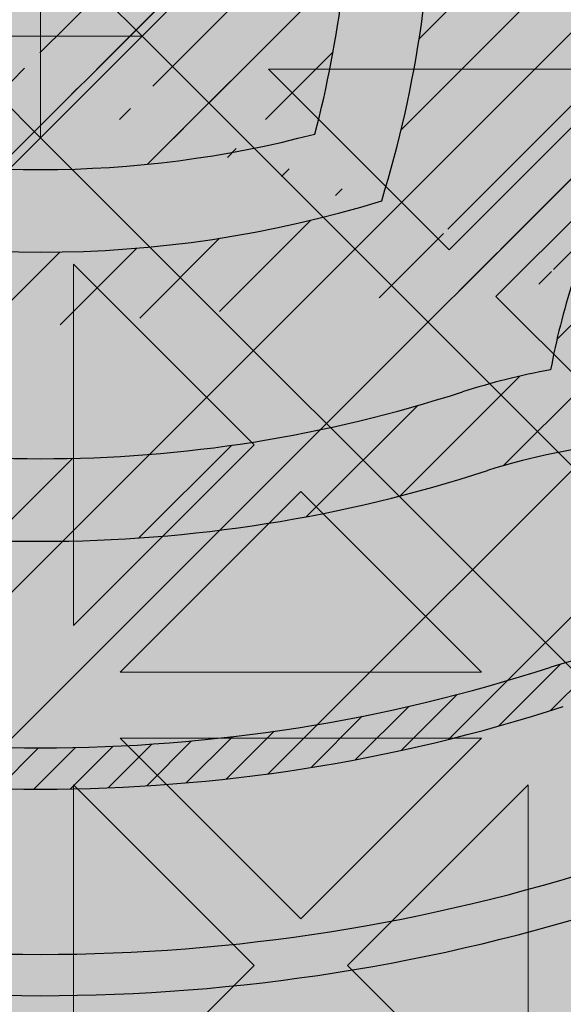
# Model space of a CAD drawing. Units: inches. Extents: x 844 to 2234, y 346 to 1084.
# Tile 54 of 93: x 1869.26 to 1871.357, y 692.527 to 696.327. Entities that reach past the tile are written whole.
import ezdxf

# ---------------------------------------------------------------- set-up
doc = ezdxf.new("R2010")
doc.units = ezdxf.units.IN
doc.header["$MEASUREMENT"] = 0
doc.layers.add('furniture', color=8, linetype='Continuous', lineweight=18)
doc.layers.add('RA-AP-01$0$INT', color=35, linetype='Continuous', lineweight=5)
doc.layers.add('RA-AP-01$0$FURN', color=3, linetype='Continuous')
doc.layers.add('RA-AP-01$0$WOOD', color=64, linetype='Continuous')

# ---------------------------------------------------------------- blocks, each defined once
blk = doc.blocks.new('A$C18D01794')
at = {"layer": 'RA-AP-01$0$INT'}
h = blk.add_hatch(color=256, dxfattribs=at)
h.paths.add_polyline_path([(4.585917135068449, -6.356712009588271), (4.555206456959269, -6.35671200958746), (4.555206456959137, -6.387422687716308), (4.874495778835233, -6.706712009592356), (4.90520645695423, -6.676001331474049)])
h.paths.add_polyline_path([(5.255206456948813, -6.387422687716306), (5.255206456948682, -6.356712009605972), (5.224495778822613, -6.356712009605161), (4.905206456953498, -6.676001331474273), (4.935917135072151, -6.706712009592924)])
h.paths.add_polyline_path([(4.935917135072559, -6.706712009592068), (4.905206456953564, -6.737422687710376), (5.255206456951813, -7.087422687708613), (5.255206456951549, -7.026001331471008)])
h.paths.add_polyline_path([(4.555206456956399, -7.026001331471013), (4.555206456956134, -7.087422687708616), (4.905206456953821, -6.737422687710943), (4.874495778835166, -6.70671200959229)])
h = blk.add_hatch(color=256, dxfattribs=at)
h.paths.add_polyline_path([(4.585917135068448, -6.356712009588273), (4.614201406330596, -6.356712009589021), (4.668846067270487, -6.411356670531338), (4.723490728212344, -6.356712009591912), (4.771774999457151, -6.35671200959319), (4.826419660396886, -6.411356670535356), (4.862780050090322, -6.374996280843536), (4.844495778842715, -6.356712009595112), (4.862780050090411, -6.356712009595595), (4.905206456960182, -6.399138416468211), (4.947632863832445, -6.356712009597838), (4.965917135079675, -6.356712009598322), (4.947632863831759, -6.374996280845421), (4.983993253523576, -6.411356670538857), (5.038637914464627, -6.356712009600247), (5.08692218571208, -6.356712009601523), (5.141566846649976, -6.411356670541852), (5.196211507589851, -6.356712009604411), (5.224495778822615, -6.356712009605161), (4.905206456953975, -6.676001331473793)])
h.paths.add_polyline_path([(4.895206456956031, -6.637717060225675), (4.895206456958921, -6.528427738347902), (4.840561796018589, -6.583072399285802)], flags=16)
h.paths.add_polyline_path([(4.915206456955638, -6.637717060226121), (4.969851117895509, -6.583072399288678), (4.915206456957609, -6.528427738348344)], flags=16)
h.paths.add_polyline_path([(4.826419660395175, -6.568930263661755), (4.881064321335613, -6.514285602723745), (4.771774999456703, -6.514285602720857)], flags=16)
h.paths.add_polyline_path([(4.983993253519558, -6.568930263665262), (5.038637914460456, -6.514285602726792), (4.929348592581548, -6.514285602724816)], flags=16)
h.paths.add_polyline_path([(4.881064321336025, -6.494285602723742), (4.826419660397532, -6.439640941782821), (4.771774999457062, -6.494285602720859)], flags=16)
h.paths.add_polyline_path([(4.929348592582019, -6.494285602724817), (5.038637914460982, -6.494285602726792), (4.983993253522945, -6.439640941786327)], flags=16)
h.paths.add_polyline_path([(4.895206456960191, -6.480143467100443), (4.895206456962115, -6.407422687715913), (4.876922185715016, -6.389138416467584), (4.840561796021581, -6.425498806159401)], flags=16)
h.paths.add_polyline_path([(4.915206456958487, -6.480143467100889), (4.969851117899527, -6.425498806162279), (4.933490728206909, -6.389138416468043), (4.9152064569598, -6.40742268771434)], flags=16)
h.paths.add_polyline_path([(4.757632863832376, -6.480143467096812), (4.812277524772842, -6.425498806158772), (4.757632863834348, -6.370854145217844)], flags=16)
h.paths.add_polyline_path([(4.737632863832376, -6.480143467096286), (4.737632863834348, -6.370854145217375), (4.682988202893906, -6.425498806155385)], flags=16)
h.paths.add_polyline_path([(5.05278005008503, -6.480143467103376), (5.052780050087917, -6.370854145224413), (4.998135389146995, -6.425498806162908)], flags=16)
h.paths.add_polyline_path([(5.072780050085024, -6.480143467103744), (5.127424711025931, -6.42549880616527), (5.072780050087916, -6.370854145224832)], flags=16)
h.paths.add_polyline_path([(4.935917135072783, -6.706712009592292), (5.255206456948811, -6.387422687716309), (5.255206456948932, -6.415706958964177), (5.200561796010279, -6.470351619902839), (5.255206456949403, -6.524996280841948), (5.25520645694961, -6.5732805520894), (5.200561796009787, -6.627925213029239), (5.236922185702417, -6.664285602721864), (5.255206456949919, -6.646001331474357), (5.255206456949998, -6.664285602721898), (5.212780050078687, -6.706712009592262), (5.25520645695036, -6.749138416463932), (5.255206456950438, -6.767422687711313), (5.236922185702424, -6.749138416463297), (5.200561796009796, -6.785498806155928), (5.255206456950753, -6.840143467096874), (5.25520645695096, -6.888427738341682), (5.200561796010322, -6.943072399282328), (5.255206456951428, -6.997717060223427), (5.255206456951547, -7.026001331471006)])
h.paths.add_polyline_path([(5.042988202883395, -6.785498806155427), (5.097632863823085, -6.840143467095101), (5.097632863822622, -6.730854145216193)], flags=16)
h.paths.add_polyline_path([(5.028846067259663, -6.771356670531693), (5.083490728198774, -6.716712009592573), (4.974201406321001, -6.716712009593042)], flags=16)
h.paths.add_polyline_path([(5.117632863823087, -6.840143467095186), (5.172277524762331, -6.785498806155926), (5.11763286382262, -6.730854145216225)], flags=16)
h.paths.add_polyline_path([(5.08349072819877, -6.696712009593886), (5.028846067259652, -6.642067348654775), (4.974201406320998, -6.696712009593438)], flags=16)
h.paths.add_polyline_path([(5.131774999446817, -6.854285602718917), (5.186419660386065, -6.799640941779662), (5.241064321325782, -6.854285602719365)], flags=17)
h.paths.add_polyline_path([(5.131774999446228, -6.716712009592374), (5.186419660386065, -6.771356670532194), (5.222780050079488, -6.734996280838764), (5.204495778832781, -6.716712009592063)], flags=16)
h.paths.add_polyline_path([(5.097632863822613, -6.682569873970264), (5.097632863823061, -6.573280552091354), (5.042988202883383, -6.627925213031044)], flags=16)
h.paths.add_polyline_path([(5.131774999446899, -6.874285602718915), (5.241064321325809, -6.874285602719364), (5.186419660386591, -6.928930263658598)], flags=17)
h.paths.add_polyline_path([(5.131774999446226, -6.696712009594078), (5.204495778830767, -6.696712009594374), (5.22278005007868, -6.67842773834687), (5.186419660386049, -6.642067348654249)], flags=16)
h.paths.add_polyline_path([(5.11763286382262, -6.682569873970225), (5.17227752476232, -6.627925213030515), (5.117632863823064, -6.573280552091267)], flags=16)
h.paths.add_polyline_path([(5.186419660386069, -6.613783077405491), (5.241064321325754, -6.559138416465795), (5.131774999446791, -6.559138416466263)], flags=16)
h.paths.add_polyline_path([(5.131774999446872, -6.539138416466263), (5.24106432132578, -6.539138416465794), (5.186419660386554, -6.484493755526573)], flags=16)
h.paths.add_polyline_path([(5.255206456951811, -7.08742268770861), (5.255206456951895, -7.106712009588038), (4.555206456956052, -7.106712009588038), (4.555206456956136, -7.087422687708617), (4.905206456953973, -6.737422687710788)])
h.paths.add_polyline_path([(4.983993253513404, -6.8444937555241), (4.92934859257295, -6.899138416462108), (5.03863791445186, -6.899138416465014)], flags=16)
h.paths.add_polyline_path([(4.969851117889988, -6.83035161990006), (4.915206456952556, -6.775706958960171), (4.915206456949648, -6.884996280837944)], flags=16)
h.paths.add_polyline_path([(4.929348592572535, -6.919138416462105), (4.983993253511019, -6.973783077403037), (5.038637914451496, -6.919138416465012)], flags=16)
h.paths.add_polyline_path([(5.052780050074912, -6.93328055208906), (4.998135389134438, -6.987925213027088), (5.052780050072919, -7.042569873968025)], flags=16)
h.paths.add_polyline_path([(5.07278005007491, -6.933280552089588), (5.072780050072918, -7.042569873968497), (5.127424711013374, -6.987925213030498)], flags=16)
h.paths.add_polyline_path([(4.89520645695295, -6.775706958959721), (4.840561796013067, -6.830351619897157), (4.895206456950961, -6.884996280837494)], flags=16)
h.paths.add_polyline_path([(4.915206456948365, -6.933280552085403), (4.915206456946434, -7.006001331471951), (4.933490728192729, -7.024285602719066), (4.969851117886972, -6.987925213026453)], flags=16)
h.paths.add_polyline_path([(4.881064321327021, -6.899138416461022), (4.82641966038902, -6.84449375552057), (4.771774999448108, -6.899138416459029)], flags=16)
h.paths.add_polyline_path([(4.895206456950073, -6.933280552084951), (4.840561796009022, -6.987925213023558), (4.876922185700835, -7.024285602716997), (4.895206456948749, -7.006001331469487)], flags=16)
h.paths.add_polyline_path([(4.983993253510392, -7.0020673486505), (4.947632863816944, -7.038427738342319), (4.965917135064043, -7.05671200959023), (5.038637914448995, -7.056712009591555)], flags=16)
h.paths.add_polyline_path([(4.881064321326543, -6.91913841646102), (4.771774999447578, -6.919138416459031), (4.826419660385607, -6.973783077399508)], flags=16)
h.paths.add_polyline_path([(4.905206456946447, -7.014285602717636), (4.862780050074785, -7.056712009588352), (4.947632863816685, -7.056712009589775)], flags=16)
h.paths.add_polyline_path([(5.14156684663679, -7.002067348654549), (5.086922185696452, -7.056712009592438), (5.196211507574223, -7.056712009594425)], flags=16)
h.paths.add_polyline_path([(4.8264196603837, -7.002067348646972), (4.771774999442643, -7.056712009585575), (4.8444957788276, -7.056712009587508), (4.862780050075511, -7.038427738340416)], flags=16)
h.paths.add_polyline_path([(4.812277524760289, -6.98792521302292), (4.757632863822258, -6.933280552082447), (4.757632863819352, -7.042569873961408)], flags=16)
h.paths.add_polyline_path([(4.73763286382226, -6.933280552082079), (4.682988202881349, -6.987925213020536), (4.737632863819352, -7.04256987396099)], flags=16)
h.paths.add_polyline_path([(4.723490728195188, -7.056712009584289), (4.668846067257299, -7.002067348643949), (4.614201406317417, -7.056712009581383)], flags=16)
h.paths.add_polyline_path([(4.597632863829262, -6.706712009592262), (4.555206456957951, -6.664285602721896), (4.555206456958029, -6.646001331474357), (4.573490728205535, -6.664285602721864), (4.609851117898167, -6.627925213029238), (4.555206456958338, -6.573280552089402), (4.555206456958546, -6.524996280841952), (4.60985111789767, -6.470351619902839), (4.555206456959015, -6.415706958964177), (4.555206456959138, -6.387422687716309), (4.874495778835167, -6.70671200959229), (4.5552064569564, -7.026001331471015), (4.555206456956523, -6.997717060223433), (4.609851117897629, -6.94307239928233), (4.555206456956988, -6.888427738341681), (4.555206456957198, -6.840143467096881), (4.609851117898153, -6.78549880615593), (4.573490728205528, -6.749138416463297), (4.555206456957507, -6.76742268771132), (4.555206456957585, -6.749138416463933)])
h.paths.add_polyline_path([(4.712780050085332, -6.730854145216195), (4.712780050084863, -6.840143467095105), (4.767424711024555, -6.785498806155427)], flags=16)
h.paths.add_polyline_path([(4.726922185709173, -6.716712009592573), (4.781566846648288, -6.771356670531693), (4.836211507586949, -6.716712009593043)], flags=16)
h.paths.add_polyline_path([(4.692780050085327, -6.730854145216225), (4.638135389145619, -6.785498806155928), (4.692780050084865, -6.840143467095185)], flags=16)
h.paths.add_polyline_path([(4.726922185709182, -6.696712009593886), (4.836211507586949, -6.696712009593436), (4.7815668466483, -6.642067348654773)], flags=16)
h.paths.add_polyline_path([(4.678637914461726, -6.71671200959237), (4.605917135075169, -6.716712009592063), (4.587632863828464, -6.734996280838766), (4.623993253521887, -6.771356670532195)], flags=16)
h.paths.add_polyline_path([(4.712780050085336, -6.68256987397026), (4.767424711024568, -6.627925213031042), (4.71278005008489, -6.573280552091352)], flags=16)
h.paths.add_polyline_path([(4.678637914461726, -6.696712009594076), (4.623993253521899, -6.642067348654247), (4.587632863829271, -6.67842773834687), (4.605917135077185, -6.696712009594376)], flags=16)
h.paths.add_polyline_path([(4.692780050085336, -6.682569873970228), (4.692780050084889, -6.573280552091267), (4.638135389145632, -6.627925213030515)], flags=16)
h.paths.add_polyline_path([(4.623993253521885, -6.799640941779662), (4.678637914461131, -6.854285602718915), (4.56934859258217, -6.854285602719365)], flags=17)
h.paths.add_polyline_path([(4.623993253521901, -6.613783077405509), (4.678637914461158, -6.559138416466263), (4.569348592582195, -6.559138416465795)], flags=16)
h.paths.add_polyline_path([(4.678637914461051, -6.874285602718915), (4.623993253521361, -6.928930263658598), (4.569348592582143, -6.874285602719364)], flags=17)
h.paths.add_polyline_path([(4.678637914461076, -6.539138416466263), (4.623993253521399, -6.484493755526573), (4.569348592582167, -6.539138416465796)], flags=16)
h = blk.add_hatch(color=256, dxfattribs=at)
h.paths.add_polyline_path([(4.969851117891331, -6.583072399286455), (4.915206456952669, -6.63771706022511), (4.915206456952222, -6.528427738347337)])
h.paths.add_polyline_path([(4.895206456953064, -6.637717060225108), (4.840561796014413, -6.583072399286448), (4.895206456953533, -6.528427738347335)])
h.paths.add_polyline_path([(4.826419660390684, -6.568930263662714), (4.771774999451003, -6.514285602723024), (4.881064321329913, -6.514285602723489)])
h.paths.add_polyline_path([(4.881064321329884, -6.494285602723492), (4.771774999450921, -6.494285602723024), (4.82641966039018, -6.439640941783778)])
h.paths.add_polyline_path([(4.895206456953734, -6.48014346709988), (4.840561796013912, -6.425498806160046), (4.876922185707337, -6.389138416466622), (4.895206456954043, -6.40742268771333)])
h.paths.add_polyline_path([(4.862780050082808, -6.374996280843689), (4.826419660390178, -6.411356670536314), (4.771774999450351, -6.356712009596481), (4.844495778835303, -6.356712009596181)])
h.paths.add_polyline_path([(4.812277524766446, -6.425498806160041), (4.757632863827191, -6.480143467099289), (4.757632863826741, -6.370854145220329)])
h.paths.add_polyline_path([(4.737632863827191, -6.480143467099214), (4.682988202887508, -6.425498806159518), (4.737632863826743, -6.370854145220299)])
h.paths.add_polyline_path([(4.668846067263777, -6.41135667053579), (4.614201406325123, -6.356712009597128), (4.723490728202894, -6.356712009596675)])
h.paths.add_polyline_path([(4.905206456953846, -6.399138416467422), (4.862780050082654, -6.356712009596229), (4.947632863824561, -6.356712009595756)])
h.paths.add_polyline_path([(4.915206456952028, -6.480143467099882), (4.91520645695173, -6.407422687715346), (4.933490728199234, -6.389138416467428), (4.96985111789186, -6.425498806160055)])
h.paths.add_polyline_path([(5.038637914454841, -6.494285602723048), (4.929348592575874, -6.494285602723497), (4.983993253515593, -6.439640941783787)])
h.paths.add_polyline_path([(4.983993253515065, -6.568930263662725), (4.929348592575849, -6.514285602723495), (5.038637914454755, -6.514285602723045)])
h.paths.add_polyline_path([(5.052780050079843, -6.480143467099317), (4.998135389140595, -6.425498806160058), (5.052780050080309, -6.370854145220356)])
h.paths.add_polyline_path([(4.983993253516868, -6.411356670536324), (4.947632863824241, -6.374996280843694), (4.965917135071747, -6.356712009596188), (5.038637914456701, -6.356712009596504)])
h.paths.add_polyline_path([(5.127424711019533, -6.425498806159557), (5.072780050079843, -6.480143467099239), (5.07278005008031, -6.370854145220326)])
h.paths.add_polyline_path([(5.141566846643269, -6.411356670535829), (5.086922185704154, -6.356712009596707), (5.196211507581929, -6.356712009597176)])
h = blk.add_hatch(color=256, dxfattribs=at)
h.paths.add_polyline_path([(5.028846067259997, -6.642067348655121), (4.974201406321342, -6.696712009593783), (5.083490728199115, -6.69671200959423)])
h.paths.add_polyline_path([(4.974201406321344, -6.716712009593388), (5.028846067260004, -6.771356670532039), (5.083490728199117, -6.716712009592919)])
h.paths.add_polyline_path([(5.042988202883738, -6.785498806155768), (5.097632863823428, -6.840143467095449), (5.097632863822963, -6.73085414521654)])
h.paths.add_polyline_path([(5.117632863822961, -6.730854145216568), (5.117632863823428, -6.840143467095531), (5.172277524762674, -6.785498806156272)])
h.paths.add_polyline_path([(5.131774999446572, -6.716712009592718), (5.186419660386406, -6.77135667053254), (5.222780050079831, -6.734996280839116), (5.204495778833122, -6.716712009592409)])
h.paths.add_polyline_path([(5.236922185702764, -6.749138416463644), (5.200561796010139, -6.785498806156274), (5.255206456949971, -6.840143467096101), (5.255206456950271, -6.76742268771115)])
h.paths.add_polyline_path([(5.186419660386412, -6.799640941780006), (5.131774999447164, -6.854285602719262), (5.241064321326123, -6.854285602719711)])
h.paths.add_polyline_path([(5.131774999447238, -6.874285602719261), (5.186419660386934, -6.928930263658944), (5.241064321326153, -6.874285602719709)])
h.paths.add_polyline_path([(5.200561796010663, -6.943072399282675), (5.255206456949324, -6.997717060221329), (5.255206456949777, -6.888427738343558)])
h.paths.add_polyline_path([(5.21278005007903, -6.706712009592607), (5.255206456950223, -6.749138416463798), (5.255206456950696, -6.664285602721891)])
h.paths.add_polyline_path([(5.13177499944657, -6.696712009594424), (5.204495778831106, -6.696712009594723), (5.222780050079024, -6.678427738347219), (5.186419660386397, -6.642067348654592)])
h.paths.add_polyline_path([(5.117632863823405, -6.573280552091611), (5.117632863822955, -6.682569873970578), (5.172277524762665, -6.627925213030859)])
h.paths.add_polyline_path([(5.042988202883727, -6.627925213031387), (5.097632863822957, -6.682569873970603), (5.097632863823407, -6.573280552091697)])
h.paths.add_polyline_path([(5.131774999447135, -6.559138416466609), (5.186419660386394, -6.613783077405857), (5.241064321326097, -6.559138416466144)])
h.paths.add_polyline_path([(5.200561796010128, -6.627925213029584), (5.236922185702758, -6.664285602722211), (5.255206456950264, -6.646001331474705), (5.255206456949948, -6.573280552089752)])
h.paths.add_polyline_path([(5.186419660386895, -6.484493755526919), (5.131774999447213, -6.539138416466609), (5.241064321326127, -6.539138416466142)])
h.paths.add_polyline_path([(5.200561796010624, -6.470351619903183), (5.255206456949745, -6.524996280842298), (5.255206456949276, -6.415706958964523)])
h = blk.add_hatch(color=256, dxfattribs=at)
h.paths.add_polyline_path([(4.905206456953579, -6.70671200959253), (4.905206456953751, -6.676001331474523), (4.874495778835229, -6.706712009592358)])
h.paths.add_polyline_path([(4.935917135071924, -6.706712009592703), (4.905206456953583, -6.706712009592529), (4.90520645695341, -6.737422687710532)])
h = blk.add_hatch(color=256, dxfattribs=at)
h.paths.add_polyline_path([(4.905206456953409, -6.737422687710532), (4.90520645695358, -6.706712009592529), (4.874495778835235, -6.706712009592359)])
h.paths.add_polyline_path([(4.935917135071928, -6.706712009592703), (4.905206456953754, -6.676001331474527), (4.905206456953582, -6.706712009592529)])
for p, q in [((4.905206456953975, -6.676001331473793), (4.585917135071132, -6.356712009590955)), ((4.905206456953975, -6.676001331473793), (5.224495778822613, -6.356712009605161)), ((5.052780050087917, -6.370854145224413), (4.998135389146995, -6.425498806162908)), ((5.052780050085028, -6.480143467103376), (5.052780050087917, -6.370854145224413)), ((4.935917135072783, -6.706712009592292), (5.255206456948813, -6.387422687716307)), ((4.969851117899529, -6.425498806162279), (4.93349072820771, -6.389138416468842)), ((4.9152064569598, -6.407422687715939), (4.915206456958485, -6.480143467100891)), ((4.915206456958485, -6.480143467100891), (4.969851117899529, -6.425498806162277)), ((5.052780050085028, -6.480143467103376), (4.998135389146995, -6.425498806162908)), ((4.92934859258202, -6.494285602724817), (4.983993253522945, -6.439640941786326)), ((5.038637914460983, -6.494285602726792), (4.983993253522945, -6.439640941786326)), ((5.038637914460983, -6.494285602726792), (4.92934859258202, -6.494285602724817)), ((4.929348592581546, -6.514285602724816), (4.983993253519556, -6.568930263665262)), ((5.038637914460456, -6.514285602726792), (4.929348592581546, -6.514285602724816)), ((4.983993253519558, -6.56893026366526), (5.038637914460456, -6.514285602726792)), ((4.915206456957613, -6.52842773834835), (4.969851117895507, -6.583072399288678)), ((4.915206456957609, -6.528427738348348), (4.915206456955636, -6.637717060226119)), ((5.042988202883385, -6.627925213031041), (5.097632863823062, -6.573280552091352)), ((4.915206456955636, -6.637717060226119), (4.969851117895507, -6.583072399288678)), ((5.097632863822615, -6.682569873970262), (5.042988202883383, -6.627925213031042)), ((4.974201406320999, -6.696712009593436), (5.028846067259652, -6.642067348654775)), ((5.083490728198769, -6.696712009593882), (5.028846067259652, -6.642067348654775)), ((4.874495778835233, -6.706712009592356), (4.905206456953753, -6.676001331474525)), ((4.935917135071927, -6.706712009592701), (4.905206456953751, -6.676001331474525)), ((4.905206456953753, -6.676001331474525), (4.905206456953409, -6.737422687710532)), ((5.08349072819877, -6.696712009593886), (4.974201406320999, -6.696712009593436)), ((4.874495778835233, -6.706712009592358), (4.935917135071925, -6.706712009592703)), ((4.935917135071927, -6.706712009592701), (4.905206456953407, -6.737422687710532)), ((4.935917135072783, -6.706712009592292), (5.255206456951548, -7.026001331471007))]:
    blk.add_line(p, q, dxfattribs=at)
blk = doc.blocks.new('A$C32926AE1')
at = {"layer": 'RA-AP-01$0$FURN'}
h = blk.add_hatch(dxfattribs=at)
h.set_pattern_fill('ANSI31', color=256, scale=0.1, style=0)
h.set_pattern_definition([(45, (0, 0), (-0.0088388347648318, 0.0088388347648318), [])])
edge = h.paths.add_edge_path(flags=16)
edge.add_arc((4.904771284329206, 4.246793130718756), 0.2603971832811541, 75.22398030683196, 104.7760196931204)
edge.add_arc((4.904771284329206, 4.246793130718756), 0.2603971832811541, 75.223980306832, 104.77601969312039, ccw=False)
edge = h.paths.add_edge_path(flags=16)
edge.add_arc((4.904771284329206, 4.067062675376612), 0.2603971832811541, 255.2239803068796, 284.776019693168)
edge.add_arc((4.904771284329206, 4.067062675376612), 0.2603971832811541, 255.22398030687958, 284.77601969316805, ccw=False)
edge = h.paths.add_edge_path(flags=0)
edge.add_arc((4.904771284329206, 4.067062675376612), 0.2603971832811541, 255.2239803068796, 284.776019693168)
edge.add_arc((4.904771284329206, 4.067062675376612), 0.2603971832811541, 255.22398030687958, 284.77601969316805, ccw=False)
edge = h.paths.add_edge_path(flags=0)
edge.add_arc((4.904771284329206, 4.067062675376612), 0.2603971832811541, 255.2239803068796, 284.776019693168)
edge.add_arc((4.904771284329206, 4.067062675376612), 0.2603971832811541, 255.22398030687958, 284.77601969316805, ccw=False)
edge = h.paths.add_edge_path()
edge.add_arc((4.604388392048174, 4.588829985554312), 0.1599999999999918, 342.3781640246255, 354.4317409793762)
edge.add_arc((5.090145208887507, 4.43216705527679), 0.3503971832811637, 162.0091218307731, 180.3186872093483)
edge.add_arc((5.205154176610243, 4.588829985554953), 0.1599999999999917, 185.5682590208461, 197.6218359767349)
edge.add_arc((4.904771284329229, 4.246793130718735), 0.3503971832811761, 72.00912183053516, 107.9908781690354)
edge.add_arc((9.535952835716557, 4.28682295566602), 4.798342501046485, 178.2875002453811, 181.5576802719453)
edge.add_arc((4.719397359771122, 4.43216705527679), 0.3503971832811637, 359.6813127906516, 377.9908781692269)
edge.add_arc((9.535967292294904, 4.286822350292874), 4.778371420254705, 178.2965938931842, 181.5667745797229)
edge.add_arc((4.719397359771122, 4.43216705527679), 0.3303971832811637, 359.6813127906516, 377.9908781692269)
edge.add_arc((0.2735752763637294, 4.286822350292874), 4.7783714202547, 358.4332254202771, 361.7034061068158)
edge.add_arc((5.061434214606998, 4.732549947558029), 0.1600000000000254, 252.3781640250584, 264.4317409792362)
edge.add_arc((4.748108354051257, 4.732549947558012), 0.1600000000000541, 275.5682590208426, 287.6218359759532)
edge.add_arc((4.604388392048115, 4.588829985554317), 0.1800000000000505, 342.3567572500182, 349.3735009646207)
edge.add_arc((5.205154176610254, 4.588829985554976), 0.1800000000000069, 190.6264990356027, 197.6432427513933)
edge.add_arc((5.061434214607106, 4.732549947558013), 0.1800000000000424, 252.3567572496606, 259.3735009644582)
edge.add_arc((4.904771284329208, 4.246793130718737), 0.3303971832811676, 71.99844483668534, 108.0015551637021)
edge.add_arc((4.748108354051414, 4.732549947558045), 0.1800000000000547, 280.6264990355479, 287.6432427495938)
edge.add_arc((5.090145208887514, 4.432167055276789), 0.2803971832811691, 162.8706300666893, 180.816523289902)
edge.add_arc((4.719397359771136, 4.432167055276689), 0.2803971832811534, 359.183476710103, 377.1293699333214)
edge.add_arc((4.904771284329222, 4.246793130718737), 0.2803971832811769, 72.87063006672916, 107.1293699332334)
edge.add_arc((5.090145208887522, 4.432167055276788), 0.2603971832811776, 165.2239803068007, 180.9953123810312)
edge.add_arc((4.719397359771141, 4.432167055276699), 0.2603971832811458, 359.0046876189768, 374.7760196932087)
edge.add_arc((5.090145208887507, 4.43216705527679), 0.3303971832811637, 162.0091218307731, 180.3186872093483)
edge.add_arc((9.53595427642584, 4.285015535491528), 4.728345371032053, 178.265043920078, 181.5679956281801)
edge.add_arc((0.2735882922327999, 4.285015535491582), 4.728345371032045, 358.4320043718193, 361.7349560799204)
edge.add_arc((9.535953591267507, 4.284458026472751), 4.708343996644348, 178.2573054306777, 181.5704995759608)
edge.add_arc((0.273588977391114, 4.284458026472785), 4.708343996644358, 358.4295004240388, 361.7426945693213)
edge.add_arc((0.2735889773911131, 4.029397779622582), 4.708343996644359, 358.2573054306787, 361.5704995759613)
edge.add_arc((9.535953591267518, 4.029397779622618), 4.708343996644359, 178.4295004240391, 181.7426945693223)
edge.add_arc((0.2735882922327901, 4.028840270603786), 4.728345371032054, 358.2650439200796, 361.5679956281808)
edge.add_arc((9.53595427642584, 4.028840270603841), 4.728345371032054, 178.4320043718199, 181.7349560799219)
edge.add_arc((0.2735752763637302, 4.027033455802493), 4.778371420254699, 358.2965938931842, 361.5667745797229)
edge.add_arc((4.719397359771122, 3.881688750818578), 0.3303971832811637, 342.0091218307731, 360.3186872093484)
edge.add_arc((5.090145208887507, 3.881688750818578), 0.3303971832811637, 179.6813127906516, 197.9908781692269)
edge.add_arc((9.535967292294904, 4.027033455802493), 4.778371420254705, 178.433225420277, 181.7034061068158)
edge.add_arc((4.719397359771122, 3.881688750818578), 0.3503971832811637, 342.0091218307731, 360.3186872093484)
edge.add_arc((9.53595283571655, 4.027032850429349), 4.79834250104648, 178.4423197280546, 181.7124997546188)
edge.add_arc((4.719397359771141, 3.881688750818669), 0.2603971832811458, 345.2239803067913, 360.9953123810232)
edge.add_arc((5.090145208887522, 3.88168875081858), 0.2603971832811776, 179.0046876189687, 194.7760196931993)
edge.add_arc((4.904771284329222, 4.067062675376631), 0.2803971832811769, 252.8706300667665, 287.1293699332708)
edge.add_arc((4.719397359771136, 3.881688750818678), 0.2803971832811534, 342.8706300666787, 360.8165232898969)
edge.add_arc((5.090145208887514, 3.881688750818579), 0.2803971832811691, 179.183476710098, 197.1293699333106)
edge.add_arc((4.748108354051414, 3.581305858537323), 0.1800000000000547, 72.3567572504062, 79.37350096445199)
edge.add_arc((4.904771284329208, 4.067062675376631), 0.3303971832811676, 251.9984448362979, 288.0015551633146)
edge.add_arc((5.061434214607106, 3.581305858537355), 0.1800000000000424, 100.6264990355418, 107.6432427503394)
edge.add_arc((5.205154176610254, 3.725025820540392), 0.1800000000000069, 162.3567572486066, 169.3735009643972)
edge.add_arc((4.604388392048115, 3.725025820541051), 0.1800000000000505, 10.62649903537925, 17.64324274998182)
edge.add_arc((4.748108354051257, 3.581305858537356), 0.1600000000000541, 72.37816402404681, 84.43174097915735)
edge.add_arc((4.904771284329229, 4.067062675376632), 0.3503971832811761, 252.0091218309645, 287.9908781694648)
edge.add_arc((5.061434214606998, 3.581305858537339), 0.1600000000000254, 95.56825902076373, 107.6218359749416)
edge.add_arc((5.205154176610243, 3.725025820540414), 0.1599999999999917, 162.3781640232651, 174.4317409791539)
edge.add_arc((5.090145208887507, 3.881688750818578), 0.3503971832811637, 179.6813127906516, 197.9908781692269)
edge.add_arc((4.604388392048174, 3.725025820541056), 0.1599999999999918, 5.568259020623824, 17.62183597537444)
edge.add_arc((0.2735897329420762, 4.28682295566602), 4.798342501046482, 358.4423197280547, 361.7124997546188)
edge.add_arc((0.2735897329420691, 4.027032850429348), 4.798342501046489, 358.2875002453812, 361.5576802719453)
at = {"layer": 'RA-AP-01$0$WOOD'}
h = blk.add_hatch(color=256, dxfattribs=at)
h.dxf.hatch_style = 1
h.paths.add_polyline_path([(5.157430609644524, 4.573483066760929, -0.1009492694046607), (5.155401577623758, 4.593365984175333, -0.1842662638101597), (5.172249623284174, 4.638795604568598, 0.2056608120311276), (5.179560981299304, 4.661316324430096, 0.3614336704623542), (5.134352340494423, 4.706524965234944, 0.2056608120311297), (5.111831620632933, 4.699213607219793, -0.1842662638101113), (5.066402000239693, 4.682365561559342, -0.1055311479399994), (5.045656153913092, 4.68467289944697, 0.1567636581983829), (4.763886414745334, 4.684672899446966, -0.1055311479399895), (4.743140568418733, 4.68236556155934, -0.1842662638100833), (4.6977109480255, 4.69921360721979, 0.2056608120302612), (4.675190228164109, 4.706524965234949, 0.3614336704708441), (4.629981587358889, 4.66131632442871, 0.2056608120245944), (4.637292945374126, 4.638795604567974, -0.1842662638101024), (4.654140991034615, 4.59336598417475, -0.1009492694055169), (4.652111959013835, 4.573483066760181, 0.021410119221476), (4.629748025606143, 4.156712009541676, 0.0214101192214795), (4.652111959013809, 3.739940952323101, -0.1009492694059586), (4.654140991034615, 3.720058034908448, -0.1842662638100975), (4.637292945374126, 3.674628414515226, 0.2056608120245705), (4.629981587358889, 3.652107694654492, 0.3614336704708879), (4.675190228164113, 3.606899053848249, 0.2056608120302384), (4.697710948025501, 3.614210411863408, -0.1842662638100995), (4.743140568418738, 3.63105845752386, -0.1055311479402541), (4.763886414745388, 3.628751119636215, 0.1567636581983776), (5.045656153913137, 3.628751119636244, -0.1055311479397538), (5.066402000239692, 3.631058457523857, -0.1842662638101067), (5.111831620632931, 3.614210411863407, 0.2056608120310924), (5.134352340494417, 3.606899053848256, 0.3614336704624001), (5.179560981299307, 3.652107694653103, 0.2056608120311314), (5.172249623284175, 3.6746284145146, -0.1842662638101402), (5.155401577623758, 3.72005803490786, -0.1009492694051366), (5.15743060964455, 3.739940952322354, 0.0214101192215073), (5.179794543052287, 4.156712009541468, 0.0214101192215252)])
h.paths.add_polyline_path([(4.639748609479751, 4.156712009541513, 0.0213537860821624), (4.661970494867118, 3.741887061152232, -0.094075836301374), (4.664143710413708, 3.7196126951003, -0.1824818158568985), (4.644813765429836, 3.668037719127816, 0.2056608120245319), (4.639939526753007, 3.653023905887301, 0.3614336704710246), (4.676106439397173, 3.616856993242342, 0.2056608120302234), (4.691120252638095, 3.621731231919122, -0.1824818158602558), (4.742695228611606, 3.641061176902986, -0.1029891339458722), (4.766991894714349, 3.638256818950944, 0.156709409989566), (5.042550673941472, 3.638256818950105, -0.102989133958497), (5.066847340047078, 3.641061176902949, -0.1824818158594995), (5.118422316020358, 3.621731231919103, 0.2056608120311416), (5.133436129261316, 3.616856993242346, 0.3614336704621468), (5.169603041905217, 3.653023905886178, 0.2056608120310986), (5.164728803228477, 3.668037719127177, -0.1824818158565612), (5.145398858244737, 3.719612695099578, -0.0940758363009313), (5.147572073791232, 3.741887061151398, 0.0213537860822023), (5.169793959178681, 4.156712009541451, 0.0213537860822226), (5.147572073791203, 4.571536957931898, -0.0940758363005034), (5.145398858244737, 4.59381132398362, -0.1824818158565587), (5.164728803228476, 4.645386299956021, 0.2056608120311045), (5.169603041905216, 4.66040011319702, 0.3614336704621845), (5.133436129261313, 4.696567025840856, 0.2056608120310773), (5.118422316020359, 4.691692787164098, -0.182481815859508), (5.066847340047078, 4.67236284218025, -0.1029891339584606), (5.04255067394148, 4.675167200133092, 0.156709409989566), (4.766991894714357, 4.675167200132257, -0.1029891339458842), (4.742695228611611, 4.672362842180213, -0.1824818158602725), (4.691120252638095, 4.691692787164077, 0.2056608120302152), (4.676106439397174, 4.696567025840858, 0.3614336704710363), (4.639939526753005, 4.660400113195899, 0.2056608120245495), (4.644813765429837, 4.645386299955384, -0.1824818158568934), (4.664143710413708, 4.593811323982902, -0.0940758363009187), (4.661970494867149, 4.571536957931074, 0.021353786082177)], flags=16)
h.paths.add_polyline_path([(5.129794543052235, 4.432167055276933, -0.0141661062790638), (5.130152669293814, 4.156927903047693, -0.0141661062790647), (5.129794543052234, 3.881688750818433, -0.0785247771143638), (5.10979738006795, 3.755143611847103, 0.0945969212073497), (5.105408519571111, 3.717898134952927, 0.1043170707844957), (5.116074640131521, 3.670385395016088, 0.1043170707864965), (5.068561900193738, 3.681051515576561, 0.09459692119553), (5.031316423304057, 3.676662655080835, -0.1580239521427272), (4.778226145355827, 3.676662655080367, 0.0945969211986668), (4.740980668464973, 3.681051515576592, 0.1043170707882822), (4.693467928526415, 3.670385395015844, 0.1043170707867916), (4.704134049087309, 3.717898134953662, 0.0945969211972894), (4.69974518859162, 3.755143611844042, -0.0785247771163196), (4.679748025606343, 3.881688750818406, -0.0141661062790663), (4.679389899364763, 4.156927903047693, -0.0141661062790672), (4.679748025606343, 4.432167055276998, -0.0785247771163064), (4.699745188591625, 4.55871219425134, 0.094596921197333), (4.704134049087308, 4.595957671141738, 0.1043170707867205), (4.693467928526416, 4.643470411079523, 0.1043170707882628), (4.740980668464965, 4.632804290518776, 0.0945969211988114), (4.778226145355874, 4.637193151015016, -0.158023952142669), (5.031316423304015, 4.637193151014546, 0.0945969211956361), (5.068561900193736, 4.632804290518806, 0.1043170707864979), (5.11607464013152, 4.643470411079278, 0.1043170707844617), (5.105408519571112, 4.595957671142455, 0.0945969212074597), (5.109797380067959, 4.558712194248236, -0.0785247771143467)], flags=0)
h.paths.add_polyline_path([(5.119794532311105, 4.432259799204851, -0.0142000800617244), (5.120156169157484, 4.156927903047701, -0.0142000800617277), (5.119794532311105, 3.881596006890482, -0.0784894509520253), (5.100273383573699, 3.758192358677797, 0.0940138827242913), (5.095413455884425, 3.717477693979438, 0.0606271852308753), (5.099615656341024, 3.686844378806616, 0.0606271852322524), (5.068982341167493, 3.691046579263239, 0.0940138827010453), (5.028267676478798, 3.686186651576848, -0.1580706864508061), (4.781274892180912, 3.686186651576435, 0.0940138827026903), (4.740560227491556, 3.691046579263279, 0.0606271852339895), (4.709926912317155, 3.686844378806508, 0.0606271852329405), (4.714129112773991, 3.717477693980356, 0.094013882701304), (4.709269185087677, 3.758192358669163, -0.0784894509577193), (4.689748036347473, 3.881596006890469, -0.014200080061729), (4.689386399501094, 4.156927903047709, -0.0142000800617217), (4.689748036347473, 4.432259799204808, -0.078489450957724), (4.709269185087651, 4.555663447426125, 0.0940138827014585), (4.714129112773992, 4.596378112114996, 0.0606271852329731), (4.709926912317154, 4.62701142728886, 0.0606271852340196), (4.74056022749157, 4.622809226832087, 0.0940138827024997), (4.781274892180847, 4.627669154518912, -0.1580706864508359), (5.028267676478777, 4.627669154518526, 0.0940138827010946), (5.068982341167492, 4.622809226832129, 0.060627185232254), (5.099615656341024, 4.627011427288751, 0.0606271852308727), (5.095413455884425, 4.59637811211593, 0.0940138827241088), (5.100273383573675, 4.555663447417647, -0.0784894509520978)], flags=0)
h.paths.add_polyline_path([(5.06978912287499, 4.430218106756144, -0.014241683694547), (5.070173729147532, 4.156927903047672, -0.0142416836945458), (5.06978912287499, 3.883637699339223, -0.0800609523125196), (5.052662118612511, 3.773463122773442, 0.0526421978001116), (5.04590916754064, 3.740550867606997, 0.0526421977992423), (5.012996912374707, 3.73379791653534, -0.1583028414718258), (4.796545656286308, 3.73379791653451, 0.0526421978034211), (4.763633401117837, 3.740550867607021, 0.0526421978018622), (4.756880450045755, 3.773463122774558, -0.0800609523117106), (4.739753445783639, 3.883637699339268, -0.0142416836945435), (4.739368839511098, 4.156927903047671, -0.0142416836945477), (4.739753445783639, 4.430218106756155, -0.0800609523116345), (4.75688045004574, 4.540392683320762, 0.052642197801941), (4.763633401117837, 4.573304938488346, 0.0526421978035071), (4.796545656286361, 4.580057889560873, -0.1583028414717561), (5.012996912374669, 4.580057889560039, 0.0526421977993048), (5.04590916754064, 4.57330493848837, 0.0526421978002057), (5.052662118612529, 4.540392683321868, -0.080060952312477)], flags=0)
h.paths.add_polyline_path([(5.049789715110557, 4.43038092723357, -0.0143097550741839), (5.05018085590259, 4.156927903047715, -0.0143097550741854), (5.049789715110558, 3.883474878861827, -0.0800685599149176), (5.03362098255317, 3.779581877367999, 0.0306258898956367), (5.028241146483733, 3.758218888663947, 0.0306258898977031), (5.006878157778253, 3.75283905259408, -0.1583983521624096), (4.802664410878162, 3.752839052594731, 0.0306258898946014), (4.781301422174808, 3.758218888663924, 0.0306258898967912), (4.775921586105202, 3.779581877368794, -0.080068559914251), (4.759752853548071, 3.883474878861786, -0.0143097550741854), (4.759361712756037, 4.156927903047671, -0.0143097550741854), (4.759752853548071, 4.430380927233557, -0.0800685599142479), (4.775921586105193, 4.534273928726546, 0.0306258898968306), (4.781301422174808, 4.555636917431444, 0.0306258898945754), (4.802664410878143, 4.561016753500631, -0.1583983521624168), (5.006878157778244, 4.561016753501291, 0.0306258898977177), (5.028241146483733, 4.555636917431421, 0.0306258898958182), (5.03362098255321, 4.534273928727244, -0.080068559914796)], flags=0)
h.paths.add_polyline_path([(4.999766070382627, 4.428171244713864, -0.0143443147609634), (5.000198441819402, 4.156927903047689, -0.0143443147609612), (4.999766070382627, 3.885684561381556, -0.0784641635803329), (4.987356730658798, 3.799103304488872, -0.1506053783831347), (4.822185837999821, 3.79910330448882, -0.0784641635803318), (4.809776498276007, 3.885684561381509, -0.014344314760963), (4.809344126839227, 4.156927903047677, -0.0143443147609645), (4.809776498276007, 4.428171244713873, -0.0784641635803192), (4.822185837999822, 4.514752501606549, -0.1506053783831338), (4.987356730658798, 4.514752501606494, -0.078464163580285)], flags=0)
h.paths.add_polyline_path([(4.979755254238824, 4.42764379880488, -0.0143772539198268), (4.980205517789977, 4.156927903047693, -0.0143772539198275), (4.979755254238824, 3.886212007290489, -0.0689242507424422), (4.971183264704897, 3.815276770442801, -0.1296645318904179), (4.838359303953726, 3.815276770442746, -0.0689242507424186), (4.829787314419809, 3.886212007290419, -0.0143772539198292), (4.829337050868653, 4.156927903047653, -0.0143772539198325), (4.829787314419809, 4.427643798804946, -0.0689242507424211), (4.838359303953725, 4.498579035652621, -0.1296645318904187), (4.971183264704897, 4.498579035652565, -0.0689242507424401)], flags=0)
h = blk.add_hatch(color=256, dxfattribs=at)
h.dxf.hatch_style = 1
h.paths.add_polyline_path([(5.145398858244737, 4.59381132398362, -0.1824818158565616), (5.164728803228476, 4.645386299956021, 0.2056608120311045), (5.169603041905216, 4.66040011319702, 0.3614336704621845), (5.133436129261313, 4.696567025840856, 0.2056608120310773), (5.118422316020359, 4.691692787164098, -0.182481815859508), (5.066847340047078, 4.67236284218025, -0.1029891339584606), (5.04255067394148, 4.675167200133092, 0.156709409989566), (4.766991894714357, 4.675167200132257, -0.1029891339458842), (4.742695228611611, 4.672362842180213, -0.1824818158602725), (4.691120252638095, 4.691692787164077, 0.2056608120302152), (4.676106439397174, 4.696567025840858, 0.3614336704710363), (4.639939526753005, 4.660400113195899, 0.2056608120245495), (4.644813765429837, 4.645386299955384, -0.1824818158568934), (4.664143710413708, 4.593811323982902, -0.0940758363009187), (4.661970494867149, 4.571536957931074, 0.0213537860821772), (4.639748609479751, 4.156712009541507, 0.0213537860821625), (4.661970494867119, 3.741887061152226, -0.0940758363013071), (4.664143710413708, 3.719612695100309, -0.1824818158569294), (4.644813765429836, 3.668037719127816, 0.2056608120245319), (4.639939526753007, 3.653023905887301, 0.3614336704710246), (4.676106439397173, 3.616856993242342, 0.2056608120302234), (4.691120252638095, 3.621731231919122, -0.1824818158602558), (4.742695228611606, 3.641061176902986, -0.1029891339458722), (4.766991894714349, 3.638256818950944, 0.156709409989566), (5.042550673941472, 3.638256818950105, -0.102989133958497), (5.066847340047078, 3.641061176902949, -0.1824818158594995), (5.118422316020358, 3.621731231919103, 0.2056608120311416), (5.133436129261316, 3.616856993242346, 0.3614336704621468), (5.169603041905217, 3.653023905886178, 0.2056608120310986), (5.164728803228477, 3.668037719127177, -0.1824818158565612), (5.145398858244737, 3.719612695099578, -0.0940758363009313), (5.147572073791232, 3.741887061151398, 0.0213537860822023), (5.169793959178681, 4.156712009541451, 0.0213537860822226), (5.147572073791203, 4.571536957931898, -0.0940758363004996)])
h.paths.add_polyline_path([(5.109797380067958, 4.55871219424824, -0.0785247771143472), (5.129794543052234, 4.432167055276936, -0.0141661062790644), (5.130152669293814, 4.156927903047685, -0.014166106279066), (5.129794543052234, 3.881688750818401, -0.0785247771143517), (5.109797380067946, 3.755143611847092, 0.0945969212073132), (5.105408519571111, 3.717898134952929, 0.1043170707844995), (5.116074640131521, 3.670385395016088, 0.1043170707864965), (5.068561900193738, 3.681051515576561, 0.09459692119553), (5.031316423304057, 3.676662655080835, -0.1580239521427272), (4.778226145355827, 3.676662655080367, 0.0945969211986668), (4.740980668464973, 3.681051515576592, 0.1043170707882822), (4.693467928526415, 3.670385395015844, 0.1043170707867916), (4.704134049087309, 3.717898134953662, 0.0945969211972894), (4.69974518859162, 3.755143611844042, -0.0785247771163196), (4.679748025606343, 3.881688750818406, -0.0141661062790663), (4.679389899364763, 4.156927903047693, -0.0141661062790672), (4.679748025606343, 4.432167055276998, -0.0785247771163064), (4.699745188591625, 4.55871219425134, 0.094596921197333), (4.704134049087308, 4.595957671141738, 0.1043170707867205), (4.693467928526416, 4.643470411079523, 0.1043170707882628), (4.740980668464965, 4.632804290518776, 0.0945969211988114), (4.778226145355874, 4.637193151015016, -0.158023952142669), (5.031316423304015, 4.637193151014546, 0.0945969211956361), (5.068561900193736, 4.632804290518806, 0.1043170707864979), (5.11607464013152, 4.643470411079278, 0.1043170707844617), (5.105408519571112, 4.595957671142455, 0.0945969212074504)], flags=16)
h.paths.add_polyline_path([(5.100273383573655, 4.55566344741771, -0.0784894509521388), (5.119794532311105, 4.432259799204852, -0.0142000800617252), (5.120156169157484, 4.156927903047686, -0.014200080061726), (5.119794532311105, 3.881596006890502, -0.0784894509520446), (5.100273383573696, 3.758192358677786, 0.0940138827242721), (5.095413455884425, 3.717477693979436, 0.0606271852308692), (5.099615656341024, 3.686844378806616, 0.0606271852322522), (5.068982341167493, 3.691046579263239, 0.0940138827010453), (5.028267676478798, 3.686186651576848, -0.1580706864508061), (4.781274892180912, 3.686186651576435, 0.0940138827026903), (4.740560227491556, 3.691046579263279, 0.0606271852339895), (4.709926912317155, 3.686844378806508, 0.0606271852329405), (4.714129112773991, 3.717477693980356, 0.094013882701304), (4.709269185087677, 3.758192358669163, -0.0784894509577193), (4.689748036347473, 3.881596006890469, -0.014200080061729), (4.689386399501094, 4.156927903047709, -0.0142000800617217), (4.689748036347473, 4.432259799204808, -0.078489450957724), (4.709269185087651, 4.555663447426125, 0.0940138827014585), (4.714129112773992, 4.596378112114996, 0.0606271852329731), (4.709926912317154, 4.62701142728886, 0.0606271852340196), (4.74056022749157, 4.622809226832087, 0.0940138827024997), (4.781274892180847, 4.627669154518912, -0.1580706864508359), (5.028267676478777, 4.627669154518526, 0.0940138827010946), (5.068982341167492, 4.622809226832129, 0.060627185232254), (5.099615656341024, 4.627011427288751, 0.0606271852308727), (5.095413455884425, 4.59637811211593, 0.094013882723957)], flags=0)
h.paths.add_polyline_path([(5.04590916754064, 4.57330493848837, 0.0526421978002057), (5.052662118612529, 4.540392683321868, -0.0800609523124783), (5.06978912287499, 4.430218106756142, -0.0142416836945469), (5.070173729147532, 4.156927903047672, -0.0142416836945458), (5.06978912287499, 3.883637699339223, -0.0800609523125196), (5.052662118612511, 3.773463122773442, 0.0526421978001116), (5.04590916754064, 3.740550867606997, 0.0526421977992423), (5.012996912374707, 3.73379791653534, -0.1583028414718258), (4.796545656286308, 3.73379791653451, 0.0526421978034211), (4.763633401117837, 3.740550867607021, 0.0526421978018622), (4.756880450045755, 3.773463122774558, -0.0800609523117106), (4.739753445783639, 3.883637699339268, -0.0142416836945435), (4.739368839511098, 4.156927903047671, -0.0142416836945477), (4.739753445783639, 4.430218106756155, -0.0800609523116345), (4.75688045004574, 4.540392683320762, 0.052642197801941), (4.763633401117837, 4.573304938488346, 0.0526421978035071), (4.796545656286361, 4.580057889560873, -0.1583028414717561), (5.012996912374669, 4.580057889560039, 0.0526421977993048)], flags=0)
h.paths.add_polyline_path([(5.028241146483733, 4.555636917431422, 0.0306258898956949), (5.033620982553182, 4.534273928727329, -0.0800685599148649), (5.049789715110557, 4.430380927233569, -0.0143097550741839), (5.05018085590259, 4.156927903047715, -0.0143097550741854), (5.049789715110558, 3.883474878861827, -0.0800685599149176), (5.03362098255317, 3.779581877367999, 0.0306258898956367), (5.028241146483733, 3.758218888663947, 0.0306258898977031), (5.006878157778253, 3.75283905259408, -0.1583983521624096), (4.802664410878162, 3.752839052594731, 0.0306258898946014), (4.781301422174808, 3.758218888663924, 0.0306258898967912), (4.775921586105202, 3.779581877368794, -0.080068559914251), (4.759752853548071, 3.883474878861786, -0.0143097550741854), (4.759361712756037, 4.156927903047671, -0.0143097550741854), (4.759752853548071, 4.430380927233557, -0.0800685599142479), (4.775921586105193, 4.534273928726546, 0.0306258898968306), (4.781301422174808, 4.555636917431444, 0.0306258898945754), (4.802664410878143, 4.561016753500631, -0.1583983521624168), (5.006878157778244, 4.561016753501291, 0.0306258898977174)], flags=0)
h.paths.add_polyline_path([(4.987356730658798, 4.514752501606494, -0.0784641635803018), (4.999766070382627, 4.428171244713845, -0.0143443147609637), (5.000198441819402, 4.156927903047665, -0.0143443147609622), (4.999766070382628, 3.885684561381514, -0.0784641635802952), (4.987356730658797, 3.799103304488872, -0.1506053783831338), (4.822185837999821, 3.799103304488819, -0.0784641635803342), (4.809776498276007, 3.885684561381512, -0.0143443147609628), (4.809344126839227, 4.156927903047676, -0.0143443147609646), (4.809776498276007, 4.428171244713873, -0.0784641635803192), (4.822185837999822, 4.514752501606549, -0.1506053783831338)], flags=0)
h.paths.add_polyline_path([(4.971183264704897, 4.498579035652566, -0.0689242507424384), (4.979755254238824, 4.427643798804883, -0.0143772539198276), (4.980205517789977, 4.15692790304768, -0.0143772539198258), (4.979755254238823, 3.88621200729051, -0.0689242507424628), (4.971183264704897, 3.815276770442801, -0.129664531890417), (4.838359303953726, 3.815276770442746, -0.0689242507424186), (4.829787314419809, 3.886212007290419, -0.0143772539198292), (4.829337050868653, 4.156927903047653, -0.0143772539198325), (4.829787314419809, 4.427643798804946, -0.0689242507424211), (4.838359303953725, 4.498579035652621, -0.1296645318904187)], flags=0)
h = blk.add_hatch(dxfattribs=at)
h.set_pattern_fill('ANSI31', color=256, scale=0.05, style=0)
h.set_pattern_definition([(45, (0, 0), (-0.0044194173824159, 0.0044194173824159), [])])
h.paths.add_polyline_path([(5.130152669293814, 4.156927903047704, 0.0141661062790657), (5.129794543052234, 4.432167055276982, 0.0777827904001433), (5.110168979996553, 4.557559993161921, -0.0976515123401879), (5.105408519571111, 4.595957671142454, -0.1043170707844687), (5.116074640131522, 4.64347041107928), (5.099615656341024, 4.627011427288751, 0.0606271852308727), (5.095413455884425, 4.59637811211593, 0.0940138827241088), (5.100273383573675, 4.555663447417647, -0.0784894509520972), (5.119794532311105, 4.432259799204852, -0.0142000800617252), (5.120156169157484, 4.156927903047686, -0.014200080061726), (5.119794532311105, 3.881596006890502, -0.0784894509520446), (5.100273383573696, 3.758192358677786, 0.0940138827242721), (5.095413455884425, 3.717477693979436, 0.0606271852308692), (5.099615656341024, 3.686844378806616), (5.116074640131519, 3.67038539501609, -0.1043170707844594), (5.105408519571112, 3.717898134952912, -0.0976515123401594), (5.11016897999655, 3.756295812933435, 0.0777827904001654), (5.129794543052234, 3.881688750818409, 0.0141661062790665)])
h.paths.add_polyline_path([(5.030164222210597, 3.676291055149937, -0.0976515123472002), (5.068561900193739, 3.681051515576561, -0.1043170707864927), (5.116074640131521, 3.670385395016088), (5.099615656341024, 3.686844378806616, 0.0606271852322522), (5.068982341167493, 3.691046579263239, 0.0940138827010453), (5.028267676478798, 3.686186651576848, -0.1580706864508061), (4.781274892180912, 3.686186651576435, 0.0940138827026903), (4.740560227491556, 3.691046579263279, 0.0606271852339913), (4.709926912317154, 3.686844378806508), (4.693467928526416, 3.670385395015845, -0.1043170707882796), (4.740980668464973, 3.681051515576592, -0.0976515123427246), (4.779378346446416, 3.676291055150394, 0.156512506893803)])
h.paths.add_polyline_path([(4.689748036347473, 3.881596006890472, -0.014200080061729), (4.689386399501094, 4.156927903047712, -0.0142000800617195), (4.689748036347473, 4.432259799204768, -0.078489450957742), (4.709269185087648, 4.555663447426114, 0.0940138827014821), (4.714129112773992, 4.596378112114995, 0.0606271852329748), (4.709926912317154, 4.62701142728886), (4.693467928526414, 4.643470411079524, -0.1043170707867939), (4.704134049087309, 4.595957671141706, -0.09765151234893), (4.699373588660725, 4.557559993157876, 0.0777827903975372), (4.679748025606343, 4.432167055276987, 0.0141661062790675), (4.679389899364763, 4.156927903047675, 0.0141661062790641), (4.679748025606343, 3.88168875081843, 0.0777827903975637), (4.699373588660724, 3.756295812937497, -0.0976515123490278), (4.704134049087308, 3.717898134953629, -0.1043170707867196), (4.693467928526416, 3.670385395015845), (4.709926912317155, 3.686844378806508, 0.0606271852329413), (4.714129112773991, 3.717477693980357, 0.0940138827013084), (4.709269185087676, 3.758192358669166, -0.0784894509577192)])
h.paths.add_polyline_path([(4.779378346446434, 4.63756475094498, -0.0976515123427943), (4.740980668464964, 4.632804290518776, -0.1043170707882609), (4.693467928526416, 4.643470411079523), (4.709926912317154, 4.62701142728886, 0.0606271852340196), (4.74056022749157, 4.622809226832087, 0.0940138827024997), (4.781274892180847, 4.627669154518912, -0.1580706864508359), (5.028267676478777, 4.627669154518526, 0.0940138827010946), (5.068982341167492, 4.622809226832129, 0.060627185232254), (5.099615656341024, 4.627011427288751), (5.116074640131521, 4.643470411079279, -0.1043170707865022), (5.068561900193735, 4.632804290518806, -0.0976515123475899), (5.030164222210446, 4.637564750945479, 0.1565125068936924)])
h = blk.add_hatch(dxfattribs=at)
h.set_pattern_fill('ANSI32', color=256, scale=0.2, style=0)
h.set_pattern_definition([(45, (0, 0), (-0.0530330085889911, 0.0530330085889911), []), (45, (0.035355339, 0), (-0.0530330085889911, 0.0530330085889911), [])])
h.paths.add_polyline_path([(5.119794532311105, 4.432259799204823, 0.0777015974868765), (5.10065834347252, 4.554469821747928, -0.0968902511992216), (5.095413455884425, 4.596378112115931, -0.060627185230871), (5.099615656341024, 4.627011427288751, -0.060627185232254), (5.068982341167492, 4.622809226832129, -0.0968902512198245), (5.027074050790956, 4.628054114423209, 0.1564657949319105), (4.782468517866163, 4.628054114422785, -0.0968902512152247), (4.740560227491555, 4.622809226832088, -0.0606271852339878), (4.709926912317155, 4.627011427288859, -0.0606271852329413), (4.714129112773991, 4.596378112115011, -0.0968902512205338), (4.708884225182929, 4.554469821738175, 0.0777015974804443), (4.689748036347473, 4.43225979920482, 0.0142000800617215), (4.689386399501094, 4.156927903047726, 0.0142000800617273), (4.689748036347473, 3.88159600689052, 0.077701597480541), (4.708884225182985, 3.759385984357019, -0.096890251220082), (4.714129112773992, 3.717477693980371, -0.0606271852329731), (4.709926912317154, 3.686844378806507, -0.060627185233988), (4.740560227491554, 3.691046579263279, -0.0968902512152569), (4.782468517866175, 3.685801691672578, 0.1564657949319236), (5.027074050790988, 3.685801691672169, -0.0968902512197451), (5.068982341167491, 3.691046579263239, -0.0606271852322557), (5.099615656341024, 3.686844378806616, -0.0606271852308727), (5.095413455884425, 3.717477693979438, -0.0968902511991229), (5.100658343472507, 3.7593859843474, 0.0777015974868745), (5.119794532311105, 3.8815960068905, 0.014200080061726), (5.120156169157484, 4.156927903047685, 0.0142000800617238)])
h.paths.add_polyline_path([(5.070173729147531, 4.156927903047684, -0.0142416836945481), (5.06978912287499, 3.883637699339191, -0.0800609523125107), (5.052662118612505, 3.773463122773424, 0.0526421978000811), (5.04590916754064, 3.740550867606997, 0.0526421977993214), (5.012996912374658, 3.733797916535325, -0.1583028414717916), (4.796545656286304, 3.733797916534512, 0.0526421978034138), (4.763633401117837, 3.740550867607021, 0.0526421978018622), (4.756880450045755, 3.773463122774558, -0.0800609523117106), (4.739753445783639, 3.883637699339268, -0.0142416836945435), (4.739368839511098, 4.156927903047671, -0.0142416836945477), (4.739753445783639, 4.430218106756155, -0.0800609523116345), (4.75688045004574, 4.540392683320762, 0.052642197801941), (4.763633401117837, 4.573304938488346, 0.0526421978035071), (4.796545656286361, 4.580057889560873, -0.1583028414717561), (5.012996912374669, 4.580057889560039, 0.0526421977993048), (5.04590916754064, 4.57330493848837, 0.0526421978002057), (5.052662118612529, 4.540392683321868, -0.0800609523124783), (5.06978912287499, 4.430218106756142, -0.0142416836945463)], flags=16)
h.paths.add_polyline_path([(5.050180855902591, 4.156927903047686, -0.0143097550741856), (5.049789715110558, 3.883474878861795, -0.0800685599148126), (5.033620982553202, 3.7795818773681, 0.0306258898957837), (5.028241146483733, 3.758218888663947, 0.0306258898977031), (5.006878157778253, 3.75283905259408, -0.1583983521624096), (4.802664410878162, 3.752839052594731, 0.0306258898946014), (4.781301422174808, 3.758218888663924, 0.0306258898967912), (4.775921586105202, 3.779581877368794, -0.080068559914251), (4.759752853548071, 3.883474878861786, -0.0143097550741854), (4.759361712756037, 4.156927903047671, -0.0143097550741854), (4.759752853548071, 4.430380927233557, -0.0800685599142479), (4.775921586105193, 4.534273928726546, 0.0306258898968306), (4.781301422174808, 4.555636917431444, 0.0306258898945754), (4.802664410878143, 4.561016753500631, -0.1583983521624168), (5.006878157778244, 4.561016753501291, 0.0306258898977177), (5.028241146483733, 4.555636917431421, 0.0306258898958182), (5.03362098255321, 4.534273928727244, -0.0800685599147973), (5.049789715110557, 4.430380927233568, -0.0143097550741854)], flags=0)
h.paths.add_polyline_path([(5.000198441819402, 4.15692790304769, -0.0143443147609622), (4.999766070382627, 3.885684561381539, -0.0784641635803169), (4.987356730658798, 3.799103304488873, -0.1506053783831347), (4.822185837999821, 3.79910330448882, -0.0784641635803318), (4.809776498276007, 3.885684561381509, -0.014344314760963), (4.809344126839227, 4.156927903047677, -0.0143443147609645), (4.809776498276007, 4.428171244713873, -0.0784641635803192), (4.822185837999822, 4.514752501606549, -0.1506053783831338), (4.987356730658798, 4.514752501606494, -0.0784641635803018), (4.999766070382627, 4.428171244713845, -0.0143443147609624)], flags=0)
h.paths.add_polyline_path([(4.980205517789976, 4.156927903047707, -0.0143772539198295), (4.979755254238824, 3.886212007290466, -0.06892425074242), (4.971183264704897, 3.815276770442801, -0.129664531890417), (4.838359303953726, 3.815276770442746, -0.0689242507424186), (4.829787314419809, 3.886212007290419, -0.0143772539198292), (4.829337050868653, 4.156927903047653, -0.0143772539198325), (4.829787314419809, 4.427643798804946, -0.0689242507424211), (4.838359303953725, 4.498579035652621, -0.1296645318904187), (4.971183264704897, 4.498579035652565, -0.0689242507424418), (4.979755254238824, 4.427643798804878, -0.0143772539198259)], flags=0)
for centre, radius, start, end in [((4.719397359771141, 3.881688750818669), 0.2603971832811458, 345.2239803067913, 0.9953123810231653), ((4.719397359771136, 3.881688750818678), 0.2803971832811534, 342.8706300666787, 0.8165232898969792), ((4.904771284329206, 4.067062675376612), 0.2603971832811541, 255.2239803068796, 284.776019693168), ((4.904771284329206, 4.067062675376612), 0.2603971832811541, 255.2239803068796, 284.776019693168), ((4.904771284329222, 4.067062675376631), 0.2803971832811769, 252.8706300667665, 287.1293699332708), ((5.205154176610254, 3.725025820540392), 0.1800000000000069, 162.3567572486066, 169.3735009643972), ((5.061434214607106, 3.581305858537355), 0.1800000000000424, 100.6264990355418, 107.6432427503394), ((4.904771284329208, 4.067062675376631), 0.3303971832811676, 251.9984448362979, 288.0015551633146), ((5.061434214606998, 3.581305858537339), 0.1600000000000254, 95.56825902076373, 107.6218359749416), ((4.904771284329229, 4.067062675376632), 0.3503971832811761, 252.0091218309645, 287.9908781694648), ((5.061434214607086, 3.581305858537378), 0.1100000000000147, 86.06530991086065, 107.5485591618349), ((4.904771284329219, 4.067062675376634), 0.4003971832811741, 252.0350753990311, 287.9649246011635), ((4.904771284329219, 4.067062675376636), 0.4103971832811756, 252.0403002450644, 287.9596997551364), ((4.904771284329217, 4.067062675376635), 0.4503971832811742, 252.0623235132636, 287.9376764870612), ((4.904771284329219, 4.067062675376637), 0.4603971832811766, 252.0683908477148, 287.9316091522846)]:
    blk.add_arc(centre, radius, start, end, dxfattribs=at)
blk = doc.blocks.new('A$C5D2F253E')
at = {"layer": 'RA-AP-01$0$FURN', "xscale": -0.7999999999883585, "yscale": 0.7999999999883585, "zscale": 0.8, "rotation": 90}
blk.add_blockref('A$C18D01794', (-5.687757199772477, 4.75791982714071), dxfattribs=at)
at = {"layer": 'RA-AP-01$0$WOOD', "rotation": 270}
blk.add_blockref('A$C32926AE1', (-4.161339601644158, 5.73852594588169), dxfattribs=at)

msp = doc.modelspace()

# ---------------------------------------------------------------- block references
at = {"layer": 'furniture', "xscale": 15.94108302203742, "yscale": 15.94108302203742, "zscale": 15.94108302203742, "rotation": 90}
msp.add_blockref('A$C5D2F253E', (1882.631064852549, 701.4028671565849), dxfattribs=at)

doc.saveas('drawing.dxf')
